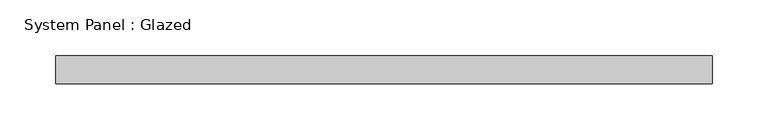
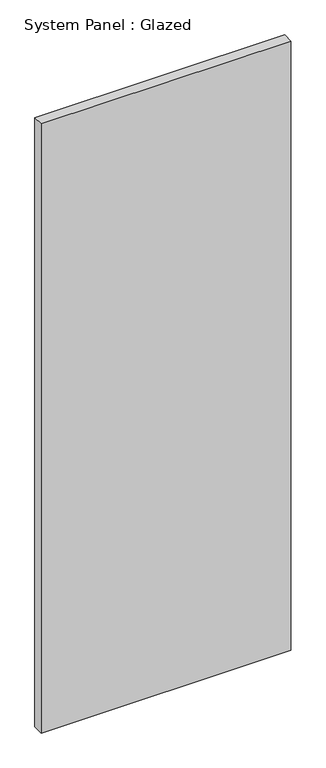
"""IFC4 building model written with IfcOpenShell, lengths in millimetres: plate geometry, System Panel : Glazed."""

from ifc_helpers import new_model, si_unit, origin, origin_with_axes, place, context, project, spatial, polyline, outline, extrude, source, transform, mapped, element, save


def system_panel_glazed_817050b2(model_context):
    return source(origin(), model_context, "Body", "SweptSolid", [
        extrude(outline(polyline([(295.275, 19.05), (-295.275, 19.05), (-295.275, 44.45), (295.275, 44.45), (295.275, 19.05)])), origin_with_axes(), (0.0, 0.0, 1.0), 1524.0),
    ])


if __name__ == "__main__":
    model = new_model("IFC4")
    model_context = context("Model", 3, world=origin())
    ifc_project = project(units=[si_unit("LENGTHUNIT", "METRE", prefix="MILLI")], contexts=[model_context])
    site = spatial("IfcSite", under=ifc_project)
    building = spatial("IfcBuilding", under=site)
    placement = place(None, origin())
    system_panel_glazed_shape = system_panel_glazed_817050b2(model_context)
    element("IfcPlate", 1, ObjectType="System Panel : Glazed", at=placement, inside=building, context=model_context, shape_type="MappedRepresentation", body=[
        mapped(system_panel_glazed_shape, transform((0.0, 0.0, 0.0), x_axis=(1.0, 0.0, 0.0), y_axis=(0.0, 1.0, 0.0), z_axis=(0.0, 0.0, 1.0))),
    ])
    save(model, "model.ifc")

# Revit data of these elements
# Type "System Panel : Glazed"
#   Construction Type Id = "GSP4R"
#   Analytic Construction = "1/8 in Pilkington single glazing"
#   Visual Light Transmittance = 0.9
#   Solar Heat Gain Coefficient = 0.86
#   Heat Transfer Coefficient (U) = 1.18115 BTU/(h·ft²·°F)
#   Define Thermal Properties by = 1
# Element 1 (IfcPlate, "System Panel : Glazed")
#   Materials on its faces: "Glass"
# Materials
#   "Glass": class "Glass", colour RGB 0 128 192, transparency 0.75, Description = "Soda Lime Glass", Cost = 0
